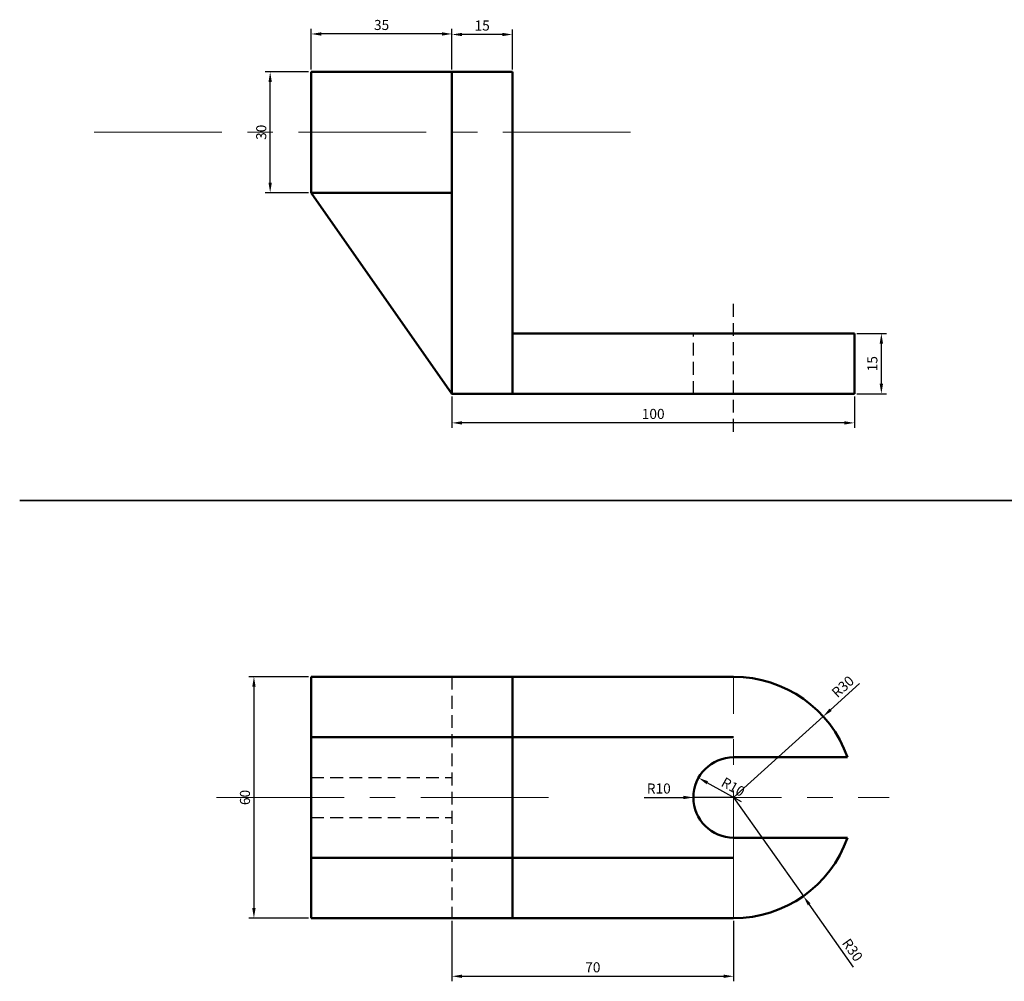
# Model space of a CAD drawing. Units: millimetres. Extents: x 2100 to 2598, y 2059 to 2386.
# Tile 1 of 1: x 2100.3 to 2345, y 2129.9 to 2368.9. Entities that reach past the tile are written whole.
import ezdxf

# ---------------------------------------------------------------- set-up
doc = ezdxf.new("R2010")
doc.units = ezdxf.units.MM
doc.linetypes.add('CENTER', pattern=[50.800000000000004, 31.75, -6.349999999999999, 6.349999999999999, -6.349999999999999])
doc.linetypes.add('HIDDEN', pattern=[9.524999999999999, 6.349999999999999, -3.174999999999999])
for name, color, linetype, lineweight in [('M-CNTR', 1, 'CENTER', 18), ('M-DIMS', 2, 'Continuous', 25), ('M-HIDN', 4, 'HIDDEN', 25), ('M-OUTL', 7, 'Continuous', 50), ('M-TTLB', 7, 'Continuous', 35)]:
    doc.layers.add(name, color=color, linetype=linetype, lineweight=lineweight)
doc.styles.get("Standard").update_dxf_attribs({"font": 'arial.ttf'})
doc.dimstyles.new('ISO-25', dxfattribs={"dimtxt": 2.5, "dimasz": 2.5, "dimexe": 1.25, "dimexo": 0.625, "dimtad": 1, "dimtxsty": 'Standard', "dimcen": 2.5, "dimadec": 0, "dimazin": 0, "dimtfac": 1, "dimtmove": 0, "dimatfit": 3, "dimfxl": 1, "dimarcsym": 0})

# ---------------------------------------------------------------- blocks, each defined once
blk = doc.blocks.new('*D10')
at = {"layer": 'Defpoints', "color": 0, "transparency": 16777216}
for p in [(2207.696528701481, 2275.948119333525), (2307.696528701481, 2275.948119333525), (2207.696528701481, 2268.730966447508)]:
    blk.add_point(p, dxfattribs=at)
at = {"layer": 'M-DIMS', "color": 0, "lineweight": -2, "transparency": 16777216}
for p, q in [((2207.696528701481, 2275.323119333525), (2207.696528701481, 2267.480966447508)), ((2307.696528701481, 2275.323119333525), (2307.696528701481, 2267.480966447508)), ((2305.196528701481, 2268.730966447508), (2210.196528701481, 2268.730966447508))]:
    blk.add_line(p, q, dxfattribs=at)
at = {"layer": 'M-DIMS', "color": 0, "transparency": 16777216}
for points in [[(2210.196528701481, 2269.147633114174), (2210.196528701481, 2268.314299780842), (2207.696528701481, 2268.730966447508)], [(2305.196528701481, 2269.147633114174), (2305.196528701481, 2268.314299780842), (2307.696528701481, 2268.730966447508)]]:
    blk.add_solid(points, dxfattribs=at)
at = {"layer": 'M-DIMS', "color": 0, "transparency": 16777216, "insert": (2257.696528701481, 2270.632398916812), "char_height": 2.5, "attachment_point": 5}
blk.add_mtext('100', dxfattribs=at)
blk = doc.blocks.new('*D11')
at = {"layer": 'Defpoints', "color": 0, "transparency": 16777216}
for p in [(2307.696528701482, 2290.948119333526), (2314.403623038992, 2290.948119333526), (2307.696528701482, 2275.948119333526)]:
    blk.add_point(p, dxfattribs=at)
at = {"layer": 'M-DIMS', "color": 0, "lineweight": -2, "transparency": 16777216}
for p, q in [((2308.321528701482, 2290.948119333526), (2315.653623038992, 2290.948119333526)), ((2314.403623038992, 2278.448119333526), (2314.403623038992, 2288.448119333526)), ((2308.321528701482, 2275.948119333526), (2315.653623038992, 2275.948119333526))]:
    blk.add_line(p, q, dxfattribs=at)
at = {"layer": 'M-DIMS', "color": 0, "transparency": 16777216}
for points in [[(2313.986956372326, 2288.448119333526), (2314.820289705659, 2288.448119333526), (2314.403623038992, 2290.948119333526)], [(2313.986956372326, 2278.448119333526), (2314.820289705659, 2278.448119333526), (2314.403623038992, 2275.948119333526)]]:
    blk.add_solid(points, dxfattribs=at)
at = {"layer": 'M-DIMS', "color": 0, "transparency": 16777216, "insert": (2312.502190569688, 2283.448119333525), "char_height": 2.5, "attachment_point": 5, "rotation": 90}
blk.add_mtext('15', dxfattribs=at)
blk = doc.blocks.new('*D12')
at = {"layer": 'Defpoints', "color": 0, "transparency": 16777216}
for p in [(2162.510380419202, 2355.948119333526), (2172.696528701482, 2355.948119333526), (2172.696528701482, 2325.948119333526)]:
    blk.add_point(p, dxfattribs=at)
at = {"layer": 'M-DIMS', "color": 0, "lineweight": -2, "transparency": 16777216}
for p, q in [((2172.071528701482, 2355.948119333526), (2161.260380419203, 2355.948119333526)), ((2162.510380419202, 2328.448119333526), (2162.510380419202, 2353.448119333526)), ((2172.071528701482, 2325.948119333526), (2161.260380419203, 2325.948119333526))]:
    blk.add_line(p, q, dxfattribs=at)
at = {"layer": 'M-DIMS', "color": 0, "transparency": 16777216}
for points in [[(2162.093713752536, 2353.448119333526), (2162.927047085869, 2353.448119333526), (2162.510380419202, 2355.948119333526)], [(2162.093713752536, 2328.448119333526), (2162.927047085869, 2328.448119333526), (2162.510380419202, 2325.948119333526)]]:
    blk.add_solid(points, dxfattribs=at)
at = {"layer": 'M-DIMS', "color": 0, "transparency": 16777216, "insert": (2160.608095289598, 2340.948119333525), "char_height": 2.5, "attachment_point": 5, "rotation": 90}
blk.add_mtext('30', dxfattribs=at)
blk = doc.blocks.new('*D13')
at = {"layer": 'Defpoints', "color": 0, "transparency": 16777216}
for p in [(2172.696528701481, 2365.395381863256), (2172.696528701481, 2355.948119333525), (2207.696528701481, 2355.948119333525)]:
    blk.add_point(p, dxfattribs=at)
at = {"layer": 'M-DIMS', "color": 0, "lineweight": -2, "transparency": 16777216}
for p, q in [((2172.696528701481, 2356.573119333525), (2172.696528701481, 2366.645381863255)), ((2207.696528701481, 2356.573119333525), (2207.696528701481, 2366.645381863255)), ((2205.196528701481, 2365.395381863256), (2175.196528701481, 2365.395381863256))]:
    blk.add_line(p, q, dxfattribs=at)
at = {"layer": 'M-DIMS', "color": 0, "transparency": 16777216}
for points in [[(2175.196528701481, 2365.812048529922), (2175.196528701481, 2364.978715196589), (2172.696528701481, 2365.395381863256)], [(2205.196528701481, 2365.812048529922), (2205.196528701481, 2364.978715196589), (2207.696528701481, 2365.395381863256)]]:
    blk.add_solid(points, dxfattribs=at)
at = {"layer": 'M-DIMS', "color": 0, "transparency": 16777216, "insert": (2190.196528701481, 2367.29766699286), "char_height": 2.5, "attachment_point": 5}
blk.add_mtext('35', dxfattribs=at)
blk = doc.blocks.new('*D14')
at = {"layer": 'Defpoints', "color": 0, "transparency": 16777216}
for p in [(2207.696528701481, 2365.263111984099), (2207.696528701481, 2355.948119333525), (2222.696528701481, 2355.948119333525)]:
    blk.add_point(p, dxfattribs=at)
at = {"layer": 'M-DIMS', "color": 0, "lineweight": -2, "transparency": 16777216}
for p, q in [((2207.696528701481, 2356.573119333525), (2207.696528701481, 2366.513111984099)), ((2222.696528701481, 2356.573119333525), (2222.696528701481, 2366.513111984099)), ((2220.196528701481, 2365.263111984099), (2210.196528701481, 2365.263111984099))]:
    blk.add_line(p, q, dxfattribs=at)
at = {"layer": 'M-DIMS', "color": 0, "transparency": 16777216}
for points in [[(2210.196528701481, 2365.679778650766), (2210.196528701481, 2364.846445317432), (2207.696528701481, 2365.263111984099)], [(2220.196528701481, 2365.679778650766), (2220.196528701481, 2364.846445317432), (2222.696528701481, 2365.263111984099)]]:
    blk.add_solid(points, dxfattribs=at)
at = {"layer": 'M-DIMS', "color": 0, "transparency": 16777216, "insert": (2215.196528701481, 2367.164544453403), "char_height": 2.5, "attachment_point": 5}
blk.add_mtext('15', dxfattribs=at)
blk = doc.blocks.new('*D18')
at = {"layer": 'Defpoints', "color": 0, "transparency": 16777216}
for p in [(2172.696528701482, 2205.638897791267), (2158.473348004203, 2145.638897791267), (2172.696528701482, 2145.638897791267)]:
    blk.add_point(p, dxfattribs=at)
at = {"layer": 'M-DIMS', "color": 0, "lineweight": -2, "transparency": 16777216}
for p, q in [((2172.071528701482, 2205.638897791267), (2157.223348004203, 2205.638897791267)), ((2158.473348004203, 2203.138897791267), (2158.473348004203, 2148.138897791266)), ((2172.071528701482, 2145.638897791267), (2157.223348004203, 2145.638897791267))]:
    blk.add_line(p, q, dxfattribs=at)
at = {"layer": 'M-DIMS', "color": 0, "transparency": 16777216}
for points in [[(2158.056681337537, 2203.138897791267), (2158.89001467087, 2203.138897791267), (2158.473348004203, 2205.638897791267)], [(2158.056681337537, 2148.138897791266), (2158.89001467087, 2148.138897791266), (2158.473348004203, 2145.638897791267)]]:
    blk.add_solid(points, dxfattribs=at)
at = {"layer": 'M-DIMS', "color": 0, "transparency": 16777216, "insert": (2156.571915534899, 2175.638897791266), "char_height": 2.5, "attachment_point": 5, "rotation": 90}
blk.add_mtext('60', dxfattribs=at)
blk = doc.blocks.new('*D19')
at = {"layer": 'Defpoints', "color": 0, "transparency": 16777216}
for p in [(2207.696528701481, 2145.638897791266), (2277.696528701481, 2145.638897791266), (2277.696528701481, 2131.198547759903)]:
    blk.add_point(p, dxfattribs=at)
at = {"layer": 'M-DIMS', "color": 0, "lineweight": -2, "transparency": 16777216}
for p, q in [((2207.696528701481, 2145.013897791266), (2207.696528701481, 2129.948547759903)), ((2277.696528701481, 2145.013897791266), (2277.696528701481, 2129.948547759903)), ((2210.196528701481, 2131.198547759903), (2275.196528701481, 2131.198547759903))]:
    blk.add_line(p, q, dxfattribs=at)
at = {"layer": 'M-DIMS', "color": 0, "transparency": 16777216}
for points in [[(2210.196528701481, 2131.615214426569), (2210.196528701481, 2130.781881093236), (2207.696528701481, 2131.198547759903)], [(2275.196528701481, 2131.615214426569), (2275.196528701481, 2130.781881093236), (2277.696528701481, 2131.198547759903)]]:
    blk.add_solid(points, dxfattribs=at)
at = {"layer": 'M-DIMS', "color": 0, "transparency": 16777216, "insert": (2242.696528701481, 2133.099980229207), "char_height": 2.5, "attachment_point": 5}
blk.add_mtext('70', dxfattribs=at)
blk = doc.blocks.new('*D20')
at = {"layer": 'Defpoints', "color": 0, "transparency": 16777216}
for p in [(2299.944734100134, 2195.76394081083), (2277.696528701481, 2175.638897791269)]:
    blk.add_point(p, dxfattribs=at)
at = {"layer": 'M-DIMS', "color": 0, "lineweight": -2, "transparency": 16777216}
for p, q in [((2309.003618551622, 2203.958329348184), (2301.798751216689, 2197.441027729126)), ((2277.696528701481, 2175.638897791269), (2299.944734100134, 2195.76394081083))]:
    blk.add_line(p, q, dxfattribs=at)
at = {"layer": 'M-DIMS', "color": 0, "transparency": 16777216}
blk.add_solid([(2301.519236730306, 2197.750030581886), (2302.078265703072, 2197.132024876368), (2299.944734100134, 2195.76394081083)], dxfattribs=at)
at = {"layer": 'M-DIMS', "color": 0, "transparency": 16777216, "insert": (2305.052074440141, 2202.948969674145), "char_height": 2.5, "attachment_point": 5, "rotation": 42.131525277352914}
blk.add_mtext('R30', dxfattribs=at)
blk = doc.blocks.new('*D21')
at = {"layer": 'Defpoints', "color": 0, "transparency": 16777216}
for p in [(2268.966618108501, 2180.516259889632), (2277.696528701483, 2175.638897791267)]:
    blk.add_point(p, dxfattribs=at)
at = {"layer": 'M-DIMS', "color": 0, "lineweight": -2, "transparency": 16777216}
blk.add_line((2279.630388500303, 2174.5584589499), (2271.149095756747, 2179.296919365041), dxfattribs=at)
at = {"layer": 'M-DIMS', "color": 0, "transparency": 16777216}
blk.add_solid([(2271.352319177512, 2179.660665639748), (2270.945872335982, 2178.933173090333), (2268.966618108501, 2180.516259889632)], dxfattribs=at)
at = {"layer": 'M-DIMS', "color": 0, "transparency": 16777216, "insert": (2277.408378418485, 2177.977952440737), "char_height": 2.5, "attachment_point": 5, "rotation": 330.80810249243603}
blk.add_mtext('R10', dxfattribs=at)
blk = doc.blocks.new('*D24')
at = {"layer": 'Defpoints', "color": 0, "transparency": 16777216}
for p in [(2277.696528999999, 2175.638898), (2295.017011999999, 2151.143983)]:
    blk.add_point(p, dxfattribs=at)
at = {"layer": 'M-DIMS', "color": 0, "lineweight": -2, "transparency": 16777216}
for p, q in [((2277.696528999999, 2175.638898), (2295.017011999999, 2151.143983)), ((2307.49215097782, 2133.501434066757), (2296.460385589579, 2149.1027400745))]:
    blk.add_line(p, q, dxfattribs=at)
at = {"layer": 'M-DIMS', "color": 0, "transparency": 16777216}
blk.add_solid([(2296.800592743828, 2149.343302339429), (2296.120178435329, 2148.86217780957), (2295.017011999999, 2151.143983)], dxfattribs=at)
at = {"layer": 'M-DIMS', "color": 0, "transparency": 16777216, "insert": (2306.962512270208, 2137.545317182767), "char_height": 2.5, "attachment_point": 5, "rotation": 305.2643312037978}
blk.add_mtext('R30', dxfattribs=at)
blk = doc.blocks.new('*D25')
at = {"layer": 'Defpoints', "color": 0, "transparency": 16777216}
for p in [(2267.696529, 2175.638999999999), (2277.696529, 2175.638897999999)]:
    blk.add_point(p, dxfattribs=at)
at = {"layer": 'M-DIMS', "color": 0, "lineweight": -2, "transparency": 16777216}
for p, q in [((2255.481317540881, 2175.639124595156), (2265.19652900013, 2175.639025499999)), ((2277.696529, 2175.638897999999), (2267.696529, 2175.638999999999))]:
    blk.add_line(p, q, dxfattribs=at)
at = {"layer": 'M-DIMS', "color": 0, "transparency": 16777216}
blk.add_solid([(2265.19653325013, 2176.055692166644), (2265.19652475013, 2175.222358833354), (2267.696529, 2175.638999999999)], dxfattribs=at)
at = {"layer": 'M-DIMS', "color": 0, "transparency": 16777216, "insert": (2259.088942665182, 2177.540520266783), "char_height": 2.5, "attachment_point": 5, "rotation": 359.9994155830492}
blk.add_mtext('R10', dxfattribs=at)

msp = doc.modelspace()

# ---------------------------------------------------------------- linework, layer by layer
at = {"layer": 'M-CNTR'}
for p, q in [((2118.749382707547, 2340.948119333525), (2258.233907020394, 2340.948119333525)), ((2277.696528701481, 2145.638897791266), (2277.696528701481, 2205.638897791266)), ((2149.160546057499, 2175.638897791266), (2234.864181375686, 2175.638897791266)), ((2257.857833881548, 2175.638897791266), (2316.351270950768, 2175.638897791266))]:
    msp.add_line(p, q, dxfattribs=at)
at = {"layer": 'M-HIDN', "ltscale": 0.5}
for p, q in [((2277.696528701481, 2266.544218713779), (2277.696528701481, 2298.42745198847)), ((2267.696528701481, 2275.948119333525), (2267.696528701481, 2290.948119333525)), ((2207.696528701481, 2205.638897791266), (2207.696528701481, 2145.638897791266)), ((2172.696528701481, 2180.638897791266), (2207.696528701481, 2180.638897791266)), ((2172.696528701481, 2170.638897791266), (2207.696528701481, 2170.638897791266))]:
    msp.add_line(p, q, dxfattribs=at)
at = {"layer": 'M-OUTL'}
for p, q in [((2207.696528701481, 2355.948119333525), (2172.696528701481, 2355.948119333525)), ((2172.696528701481, 2355.948119333525), (2172.696528701481, 2325.948119333525)), ((2222.696528701481, 2355.948119333525), (2207.696528701481, 2355.948119333525)), ((2207.696528701481, 2355.948119333525), (2207.696528701481, 2275.948119333525)), ((2222.696528701481, 2290.948119333525), (2222.696528701481, 2355.948119333525)), ((2172.696528701481, 2325.948119333525), (2207.696528701481, 2325.948119333525)), ((2172.696528701481, 2325.948119333525), (2207.696528701481, 2275.948119333525)), ((2307.696528701481, 2290.948119333525), (2222.696528701481, 2290.948119333525)), ((2222.696528701481, 2290.948119333525), (2222.696528701481, 2275.948119333525)), ((2307.696528701481, 2275.948119333525), (2307.696528701481, 2290.948119333525)), ((2207.696528701481, 2275.948119333525), (2307.696528701481, 2275.948119333525)), ((2172.696528701481, 2205.638897791266), (2172.696528701481, 2145.638897791266)), ((2242.696528701481, 2205.638897791266), (2172.696528701481, 2205.638897791266)), ((2207.696528701481, 2205.638897791266), (2277.696528701481, 2205.638897791266)), ((2222.696528701481, 2205.638897791266), (2222.696528701481, 2145.638897791266)), ((2277.69652870148, 2190.638897791266), (2172.696528701481, 2190.638897791266)), ((2277.696528701481, 2185.638897791266), (2305.980799948943, 2185.638897791266)), ((2277.696528701481, 2165.638897791266), (2305.980799948943, 2165.638897791266)), ((2172.696528701481, 2160.638897791266), (2277.69652870148, 2160.638897791266)), ((2207.696528701481, 2145.638897791266), (2172.696528701481, 2145.638897791266)), ((2207.696528701481, 2145.638897791266), (2277.696528701481, 2145.638897791266))]:
    msp.add_line(p, q, dxfattribs=at)
for radius, start, end in [(30, 19.47122063449054, 90), (10, 90, 270), (30, 270, 340.5287793655095)]:
    msp.add_arc((2277.696528701481, 2175.638897791266), radius, start, end, dxfattribs=at)
at = {"layer": 'M-TTLB'}
msp.add_line((2100.255876839101, 2249.403035994022), (2598.481187377458, 2249.403035994022), dxfattribs=at)

# ---------------------------------------------------------------- dimensions: what is measured, and where the dimension line sits
at = {"layer": 'M-DIMS'}
for p1, p2, distance, picture, middle in [((2207.696528701481, 2355.948119333525), (2172.696528701481, 2355.948119333525), -9.447262529730779, '*D13', (2190.196528701481, 2367.29766699286)), ((2222.696528701481, 2355.948119333525), (2207.696528701481, 2355.948119333525), -9.314992650573913, '*D14', (2215.196528701481, 2367.164544453403)), ((2172.696528701481, 2325.948119333525), (2172.696528701481, 2355.948119333525), 10.186148282278737, '*D12', (2160.608095289598, 2340.948119333525)), ((2307.696528701481, 2275.948119333525), (2307.696528701481, 2290.948119333525), -6.70709433751108, '*D11', (2312.502190569688, 2283.448119333525)), ((2307.696528701481, 2275.948119333525), (2207.696528701481, 2275.948119333525), 7.217152886017175, '*D10', (2257.696528701481, 2270.632398916812))]:
    dim = msp.add_aligned_dim(p1=p1, p2=p2, distance=distance, dimstyle='ISO-25', override={"dimclrd": 0, "dimclre": 0, "dimclrt": 0}, dxfattribs=at)
    dim.commit()
    dim.dimension.update_dxf_attribs({"geometry": picture, "text_midpoint": middle})
dim = msp.add_linear_dim(base=(2158.473348004203, 2145.638897791267), p1=(2172.696528701481, 2205.638897791266), p2=(2172.696528701481, 2145.638897791266), angle=90, dimstyle='ISO-25', override={"dimclrd": 0, "dimclre": 0, "dimclrt": 0}, dxfattribs=at)
dim.commit()
dim.dimension.update_dxf_attribs({"geometry": '*D18', "text_midpoint": (2156.571915534899, 2175.638897791266)})
for center, mpoint, override, picture, middle in [((2277.696528701481, 2175.638897791269), (2299.944734100134, 2195.76394081083), {"dimclrd": 0, "dimclre": 0, "dimclrt": 0}, '*D20', (2305.052074440141, 2202.948969674145)), ((2277.696529, 2175.638897999999), (2267.696529, 2175.638999999999), {"dimdec": 0, "dimlfac": 1, "dimrnd": 0, "dimzin": 0, "dimdsep": 46, "dimlunit": 2}, '*D25', (2259.088942665182, 2177.540520266783))]:
    dim = msp.add_radius_dim(center=center, mpoint=mpoint, dimstyle='ISO-25', override=override, dxfattribs=at)
    dim.commit()
    dim.dimension.update_dxf_attribs({"geometry": picture, "text_midpoint": middle})
for center, mpoint, override, picture, middle in [((2277.696528701483, 2175.638897791267), (2268.966618108501, 2180.516259889632), {"dimclrd": 0, "dimclre": 0, "dimclrt": 0}, '*D21', (2276.480980952647, 2176.318018895175)), ((2277.696528999999, 2175.638898), (2295.017011999999, 2151.143983), {"dimdec": 0, "dimlfac": 1, "dimrnd": 0, "dimzin": 0, "dimdsep": 46, "dimlunit": 2}, '*D24', (2305.409301844972, 2136.447033936399))]:
    dim = msp.add_radius_dim(center=center, mpoint=mpoint, dimstyle='ISO-25', override=override, dxfattribs=at)
    dim.commit()
    dim.dimension.update_dxf_attribs({"geometry": picture, "text_midpoint": middle, "dimtype": 164})
dim = msp.add_linear_dim(base=(2277.696528701481, 2131.198547759903), p1=(2207.696528701481, 2145.638897791266), p2=(2277.696528701481, 2145.638897791266), dimstyle='ISO-25', override={"dimclrd": 0, "dimclre": 0, "dimclrt": 0}, dxfattribs=at)
dim.commit()
dim.dimension.update_dxf_attribs({"geometry": '*D19', "text_midpoint": (2242.696528701481, 2133.099980229207)})

doc.saveas('drawing.dxf')
